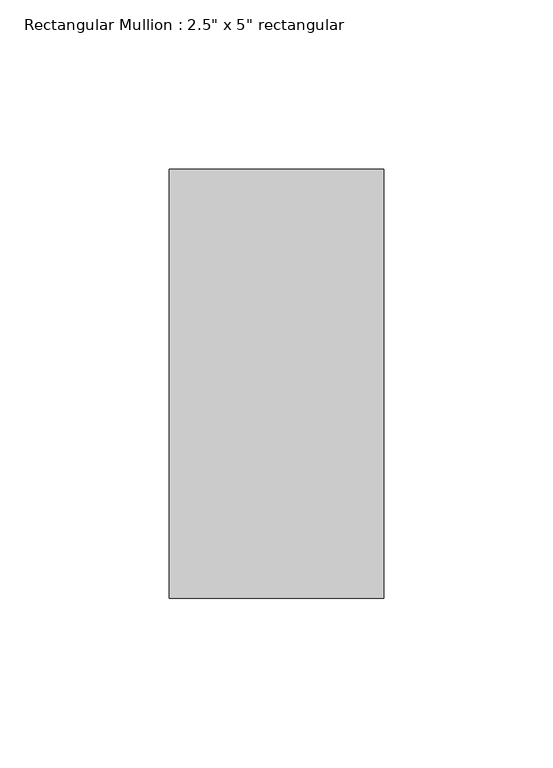
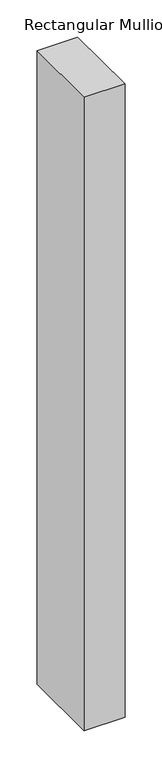
"""IFC4 building model written with IfcOpenShell, lengths in millimetres: member geometry."""

from ifc_helpers import new_model, si_unit, frame, origin, place, context, project, spatial, polyline, outline, extrude, source, transform, mapped, element, save


def member_04769ced(model_context):
    return source(origin(), model_context, "Body", "SweptSolid", [
        extrude(outline(polyline([(0.0, 63.5), (0.0, -63.5), (-63.5, -63.5), (-63.5, 63.5), (0.0, 63.5)])), frame((0.0, 0.0, -1041.8508611), z_axis=(0.0, 0.0, 1.0), x_axis=(1.0, 0.0, 0.0)), (0.0, 0.0, 1.0), 1041.8508611),
    ])


if __name__ == "__main__":
    model = new_model("IFC4")
    model_context = context("Model", 3, world=origin())
    ifc_project = project(units=[si_unit("LENGTHUNIT", "METRE", prefix="MILLI")], contexts=[model_context])
    site = spatial("IfcSite", under=ifc_project)
    building = spatial("IfcBuilding", under=site)
    placement = place(None, origin())
    member_shape = member_04769ced(model_context)
    element("IfcMember", 1, ObjectType="Rectangular Mullion : 2.5\" x 5\" rectangular", at=placement, inside=building, context=model_context, shape_type="MappedRepresentation", body=[
        mapped(member_shape, transform((0.0, 0.0, 0.0), x_axis=(1.0, 0.0, 0.0), y_axis=(0.0, 1.0, 0.0), z_axis=(0.0, 0.0, 1.0))),
    ])
    save(model, "model.ifc")

# Revit data of these elements
# Type "Rectangular Mullion : 2.5\" x 5\" rectangular"
#   built-in parameter 1007304 = 0.416667 (stored number, unit not read)
#   built-in parameter 1007301 = 0.104167 (stored number, unit not read)
#   built-in parameter 1007300 = 0.104167 (stored number, unit not read)
# Element 1 (IfcMember, "Rectangular Mullion : 2.5\" x 5\" rectangular")
#   Materials on its faces: "Aluminum"
# Materials
#   "Aluminum": class "Metal", colour RGB 247 247 247, transparency 0, Description = "Aluminum 6061", Cost = 0
